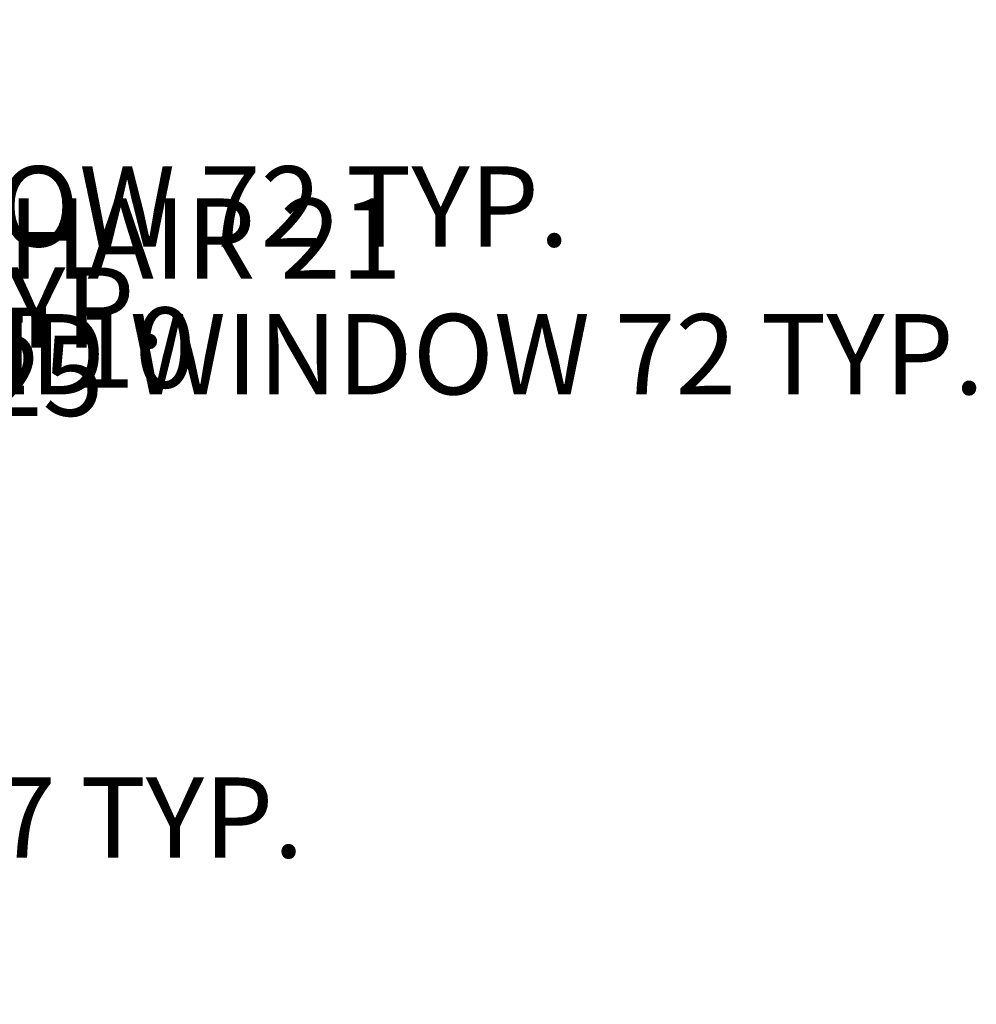
# Model space of a CAD drawing. Units: inches. Extents: x -307 to 2141, y -58 to 895.
# Tile 28 of 28: x 1283 to 2141, y -44 to 839. Entities that reach past the tile are written whole.
import ezdxf

# ---------------------------------------------------------------- set-up
doc = ezdxf.new("R2010")
doc.units = ezdxf.units.IN
doc.header["$MEASUREMENT"] = 0
doc.layers.add('A-ANNO-DIMS', color=2, linetype='Continuous', lineweight=18)
doc.styles.get("Standard").update_dxf_attribs({"font": 'arial.ttf'})
doc.dimstyles.get("Standard").update_dxf_attribs({"dimtxt": 72, "dimasz": 48, "dimexe": 0.18, "dimexo": 0.0625, "dimgap": 0.09, "dimtad": 0, "dimtih": 1, "dimtoh": 1, "dimdec": 0, "dimrnd": 48, "dimzin": 0, "dimdsep": 46, "dimlunit": 3, "dimtxsty": 'Standard', "dimcen": 0.09, "dimadec": 0, "dimazin": 0, "dimtfac": 1, "dimtdec": 0, "dimtofl": 0, "dimtmove": 0, "dimatfit": 3, "dimfxl": 1, "dimtolj": 1, "dimtzin": 0, "dimarcsym": 0})

# ---------------------------------------------------------------- blocks, each defined once
blk = doc.blocks.new('*D30')
at = {"layer": 'A-ANNO-DIMS', "color": 0, "lineweight": -2, "transparency": 16777216}
for p, q in [((570.74, 532.83), (570.74, 580.83)), ((570.74, 580.83), (618.74, 580.83)), ((565.4, 484.83), (570.92, 484.83)), ((565.4, 448.83), (570.92, 448.83)), ((570.74, 400.83), (570.74, 352.83))]:
    blk.add_line(p, q, dxfattribs=at)
at = {"layer": 'A-ANNO-DIMS', "color": 0, "transparency": 16777216}
for points in [[(562.74, 532.83), (578.74, 532.83), (570.74, 484.83)], [(562.74, 400.83), (578.74, 400.83), (570.74, 448.83)]]:
    blk.add_solid(points, dxfattribs=at)
at = {"layer": 'Defpoints', "color": 0, "transparency": 16777216}
for p in [(565.34, 484.83), (570.74, 484.83), (565.34, 448.83)]:
    blk.add_point(p, dxfattribs=at)
at = {"layer": 'A-ANNO-DIMS', "color": 0, "transparency": 16777216, "insert": (1030.17, 580.83), "char_height": 72, "attachment_point": 5}
blk.add_mtext('\\A1;WINDOW 36 TYP.', dxfattribs=at)
blk = doc.blocks.new('*D32')
at = {"layer": 'A-ANNO-DIMS', "color": 0, "lineweight": -2, "transparency": 16777216}
for p, q in [((813.29, 682.28), (813.29, 671.36)), ((885.29, 682.28), (885.29, 671.36)), ((765.29, 671.54), (717.29, 671.54)), ((933.29, 671.54), (981.29, 671.54))]:
    blk.add_line(p, q, dxfattribs=at)
at = {"layer": 'A-ANNO-DIMS', "color": 0, "transparency": 16777216}
for points in [[(765.29, 679.54), (765.29, 663.54), (813.29, 671.54)], [(933.29, 679.54), (933.29, 663.54), (885.29, 671.54)]]:
    blk.add_solid(points, dxfattribs=at)
at = {"layer": 'Defpoints', "color": 0, "transparency": 16777216}
for p in [(813.29, 682.34), (885.29, 682.34), (885.29, 671.54)]:
    blk.add_point(p, dxfattribs=at)
at = {"layer": 'A-ANNO-DIMS', "color": 0, "transparency": 16777216, "insert": (1392.73, 671.54), "char_height": 72, "attachment_point": 5}
blk.add_mtext('\\A1;WINDOW 72 TYP.', dxfattribs=at)
blk = doc.blocks.new('*D34')
at = {"layer": 'A-ANNO-DIMS', "color": 0, "lineweight": -2, "transparency": 16777216}
for p, q in [((927.14, 490.97), (927.14, 538.97)), ((927.14, 538.97), (975.14, 538.97)), ((916.4, 442.97), (927.32, 442.97)), ((916.4, 370.95), (927.32, 370.95)), ((927.14, 322.95), (927.14, 274.95))]:
    blk.add_line(p, q, dxfattribs=at)
at = {"layer": 'A-ANNO-DIMS', "color": 0, "transparency": 16777216}
for points in [[(919.14, 490.97), (935.14, 490.97), (927.14, 442.97)], [(919.14, 322.95), (935.14, 322.95), (927.14, 370.95)]]:
    blk.add_solid(points, dxfattribs=at)
at = {"layer": 'Defpoints', "color": 0, "transparency": 16777216}
for p in [(916.34, 442.97), (927.14, 442.97), (916.34, 370.95)]:
    blk.add_point(p, dxfattribs=at)
at = {"layer": 'A-ANNO-DIMS', "color": 0, "transparency": 16777216, "insert": (1584.53, 538.97), "char_height": 72, "attachment_point": 5}
blk.add_mtext('\\A1;PAIRED WINDOW 72 TYP.', dxfattribs=at)
blk = doc.blocks.new('*D40')
at = {"layer": 'A-ANNO-DIMS', "color": 0, "lineweight": -2, "transparency": 16777216}
for p, q in [((725.38, 128.89), (725.38, 123.17)), ((762.77, 128.89), (762.77, 123.17)), ((677.38, 123.35), (629.38, 123.35)), ((810.77, 123.35), (858.77, 123.35))]:
    blk.add_line(p, q, dxfattribs=at)
at = {"layer": 'A-ANNO-DIMS', "color": 0, "transparency": 16777216}
for points in [[(677.38, 131.35), (677.38, 115.35), (725.38, 123.35)], [(810.77, 131.35), (810.77, 115.35), (762.77, 123.35)]]:
    blk.add_solid(points, dxfattribs=at)
at = {"layer": 'Defpoints', "color": 0, "transparency": 16777216}
for p in [(725.38, 128.96), (762.77, 128.96), (762.77, 123.35)]:
    blk.add_point(p, dxfattribs=at)
at = {"layer": 'A-ANNO-DIMS', "color": 0, "transparency": 16777216, "insert": (1208.37, 123.35), "char_height": 72, "attachment_point": 5}
blk.add_mtext('\\A1;PLANT 37 TYP.', dxfattribs=at)
blk = doc.blocks.new('*D42')
at = {"layer": 'A-ANNO-DIMS', "color": 0, "lineweight": -2, "transparency": 16777216}
for p, q in [((774.28, 541.63), (726.29, 540.62)), ((822.3, 541.2), (822.27, 542.82)), ((832.3, 541.41), (832.27, 543.03)), ((880.26, 543.86), (928.25, 544.87))]:
    blk.add_line(p, q, dxfattribs=at)
at = {"layer": 'A-ANNO-DIMS', "color": 0, "transparency": 16777216}
for points in [[(774.11, 549.63), (774.45, 533.63), (822.27, 542.64)], [(880.09, 551.86), (880.43, 535.86), (832.27, 542.85)]]:
    blk.add_solid(points, dxfattribs=at)
at = {"layer": 'Defpoints', "color": 0, "transparency": 16777216}
for p in [(822.3, 541.14), (832.27, 542.85), (832.3, 541.35)]:
    blk.add_point(p, dxfattribs=at)
at = {"layer": 'A-ANNO-DIMS', "color": 0, "transparency": 16777216, "insert": (1192.89, 544.87), "char_height": 72, "attachment_point": 5}
blk.add_mtext('\\A1;FAUCET 10', dxfattribs=at)
blk = doc.blocks.new('*D44')
at = {"layer": 'A-ANNO-DIMS', "color": 0, "lineweight": -2, "transparency": 16777216}
for p, q in [((839.87, 521.22), (839.95, 517.42)), ((767.41, 516.08), (719.42, 515.07)), ((815.33, 520.71), (815.41, 516.91)), ((887.94, 518.61), (935.93, 519.62))]:
    blk.add_line(p, q, dxfattribs=at)
at = {"layer": 'A-ANNO-DIMS', "color": 0, "transparency": 16777216}
for points in [[(767.25, 524.08), (767.58, 508.08), (815.4, 517.09)], [(887.77, 526.61), (888.11, 510.61), (839.95, 517.6)]]:
    blk.add_solid(points, dxfattribs=at)
at = {"layer": 'Defpoints', "color": 0, "transparency": 16777216}
for p in [(839.87, 521.29), (815.33, 520.77), (839.95, 517.6)]:
    blk.add_point(p, dxfattribs=at)
at = {"layer": 'A-ANNO-DIMS', "color": 0, "transparency": 16777216, "insert": (1151.16, 519.62), "char_height": 72, "attachment_point": 5}
blk.add_mtext('\\A1;BASIN 25', dxfattribs=at)
blk = doc.blocks.new('*D46')
at = {"layer": 'A-ANNO-DIMS', "color": 0, "lineweight": -2, "transparency": 16777216}
for p, q in [((801.41, 645.78), (801.41, 642.52)), ((822.41, 645.78), (822.41, 642.52)), ((753.41, 642.7), (705.41, 642.7)), ((870.41, 642.7), (918.41, 642.7))]:
    blk.add_line(p, q, dxfattribs=at)
at = {"layer": 'A-ANNO-DIMS', "color": 0, "transparency": 16777216}
for points in [[(753.41, 650.7), (753.41, 634.7), (801.41, 642.7)], [(870.41, 650.7), (870.41, 634.7), (822.41, 642.7)]]:
    blk.add_solid(points, dxfattribs=at)
at = {"layer": 'Defpoints', "color": 0, "transparency": 16777216}
for p in [(801.41, 645.85), (822.41, 645.85), (822.41, 642.7)]:
    blk.add_point(p, dxfattribs=at)
at = {"layer": 'A-ANNO-DIMS', "color": 0, "transparency": 16777216, "insert": (1282.7, 642.7), "char_height": 72, "attachment_point": 5}
blk.add_mtext('\\A1;DESK CHAIR 21', dxfattribs=at)

msp = doc.modelspace()

# ---------------------------------------------------------------- dimensions: what is measured, and where the dimension line sits
at = {"layer": 'A-ANNO-DIMS'}
for base, p1, p2, text, picture, middle in [((885.2934, 671.5408), (813.2934, 682.3408), (885.2934, 682.3408), 'WINDOW <> TYP.', '*D32', (1392.7312, 671.5408)), ((822.4132, 642.696), (801.4132, 645.846), (822.4132, 645.846), 'DESK CHAIR <>', '*D46', (1282.7024, 642.696)), ((762.7703, 123.348), (725.3775, 128.9569), (762.7703, 128.9569), 'PLANT <> TYP.', '*D40', (1208.3746, 123.348))]:
    dim = msp.add_linear_dim(base=base, p1=p1, p2=p2, text=text, dimstyle='Standard', override={"dimdec": 0, "dimlfac": 1, "dimrnd": 0, "dimzin": 0, "dimdsep": 46, "dimlunit": 2}, dxfattribs=at)
    dim.commit()
    dim.dimension.update_dxf_attribs({"geometry": picture, "text_midpoint": middle})
for base, p1, p2, angle, text, picture, middle in [((927.1381, 442.9669), (916.3358, 370.9517), (916.3358, 442.9669), 90, 'PAIRED WINDOW <> TYP.', '*D34', (1584.5269, 538.9669)), ((570.7358, 484.8333), (565.3358, 448.8333), (565.3358, 484.8333), 90, 'WINDOW <> TYP.', '*D30', (1030.1737, 580.8333)), ((832.2692, 542.8502), (822.3029, 541.1403), (832.3007, 541.3505), 1.2046277, 'FAUCET <>', '*D42', (1192.8864, 544.8684)), ((839.9481, 517.6035), (815.3253, 520.7692), (839.8707, 521.2853), 1.2046277, 'BASIN <>', '*D44', (1151.1574, 519.6217))]:
    dim = msp.add_linear_dim(base=base, p1=p1, p2=p2, angle=angle, text=text, dimstyle='Standard', override={"dimdec": 0, "dimlfac": 1, "dimrnd": 0, "dimzin": 0, "dimdsep": 46, "dimlunit": 2}, dxfattribs=at)
    dim.commit()
    dim.dimension.update_dxf_attribs({"geometry": picture, "text_midpoint": middle})

doc.saveas('drawing.dxf')
